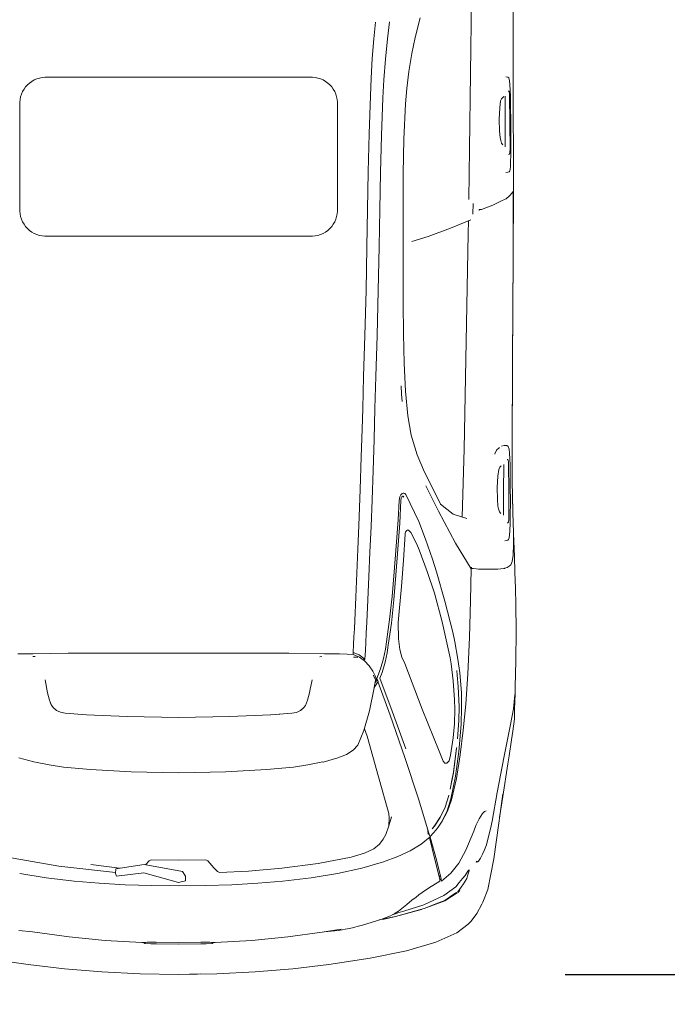
# Model space of a CAD drawing. Units: millimetres. Extents: x 595116 to 630915, y 909473 to 920225.
# Tile 6 of 134: x 629349 to 629404, y 919194 to 919279. Entities that reach past the tile are written whole.
import ezdxf

# ---------------------------------------------------------------- set-up
doc = ezdxf.new("R2010")
doc.units = ezdxf.units.MM
doc.layers.add('C-PRKG-VEHI', color=8, linetype='Continuous', lineweight=13)
doc.layers.add('Dimension', color=3, linetype='Continuous', lineweight=18)
doc.styles.get("Standard").update_dxf_attribs({"font": 'arial.ttf'})
doc.dimstyles.new('ISO-25', dxfattribs={"dimtxt": 9, "dimasz": 6, "dimexe": 1.25, "dimexo": 0.625, "dimtad": 1, "dimlunit": 4, "dimtxsty": 'Standard', "dimcen": 2.5, "dimadec": 0, "dimazin": 0, "dimtfac": 1, "dimtmove": 0, "dimatfit": 3, "dimfxl": 1, "dimarcsym": 0})

# ---------------------------------------------------------------- blocks, each defined once
blk = doc.blocks.new('A$C7ADB3080')
for p, q in [((1717.5, 1836.5), (2187.9, 1837.4)), ((2187.9, 1837.4), (2484.5, 1837.8)), ((2193.4, 1826), (2191.2, 1823.4)), ((2200.6, 1827.9), (2193.4, 1826)), ((2210.5, 1828.9), (2200.6, 1827.9)), ((2224.9, 1829.7), (2210.5, 1828.9)), ((2224.9, 1829.7), (2241, 1830)), ((2227.3, 1826.2), (2226.9, 1824.2)), ((2227.3, 1826.2), (2228.5, 1826.8)), ((2229.6, 1827.1), (2228.5, 1826.8)), ((2232.9, 1827.6), (2229.6, 1827.1)), ((2237.6, 1827.8), (2232.9, 1827.6)), ((2309.4, 1828.6), (2237.6, 1827.8)), ((2241, 1830), (2270.8, 1830.6)), ((2270.8, 1830.6), (2301.2, 1830.8)), ((2301.2, 1830.8), (2330.4, 1831.1)), ((2377.2, 1829.1), (2309.4, 1828.6)), ((2330.4, 1831.1), (2346.2, 1831.1)), ((2346.2, 1831.1), (2361.6, 1831.1)), ((2361.6, 1831.1), (2390.1, 1830.9)), ((2382.2, 1828.9), (2377.2, 1829.1)), ((2386.2, 1828.5), (2382.2, 1828.9)), ((2388.4, 1827.8), (2386.2, 1828.5)), ((2386.8, 1828.4), (2387.6, 1828.3)), ((2387.6, 1828.3), (2389.6, 1827.5)), ((2389.6, 1827.5), (2388.4, 1827.8)), ((2389.6, 1827.5), (2389.9, 1825.3)), ((2411.1, 1830.5), (2390.1, 1830.9)), ((2420.6, 1830), (2411.1, 1830.5)), ((2428.8, 1829.1), (2420.6, 1830)), ((2432.5, 1828.1), (2428.8, 1829.1)), ((2434.5, 1826.7), (2432.5, 1828.1)), ((2435.7, 1823.3), (2434.5, 1826.7)), ((2494.5, 1829.3), (2484.5, 1837.8)), ((2484.8, 1837.6), (2652.6, 1836.8)), ((2485.1, 1837.3), (2485.3, 1837.5)), ((2485.3, 1837.5), (2485.4, 1837.5)), ((2654.1, 1836.7), (2485.4, 1837.5)), ((2496.6, 1827.5), (2494.5, 1829.3)), ((2503.9, 1818.7), (2496.6, 1827.5)), ((2652.6, 1836.8), (2920.1, 1835.4)), ((2925, 1835.1), (2654.1, 1836.7)), ((3154.5, 1834.7), (2920.1, 1835.4)), ((2925, 1835.1), (3140.2, 1834.4)), ((3140.2, 1834.4), (3154.5, 1834.3)), ((3155.1, 1834.3), (3141.2, 1834.3)), ((3141.2, 1834.3), (3141.2, 1834.3)), ((3148.6, 1826.5), (3141.5, 1824)), ((3158.6, 1827.8), (3148.6, 1826.5)), ((3154.5, 1834.7), (3189.7, 1834.5)), ((3167.6, 1834.3), (3155.1, 1834.3)), ((3173, 1828.6), (3158.6, 1827.8)), ((3167.2, 1834.3), (3179.8, 1834.4)), ((3173, 1828.6), (3189, 1829)), ((3177.6, 1824.3), (3176.5, 1824)), ((3180.9, 1824.9), (3177.6, 1824.3)), ((3179.8, 1834.4), (3189.8, 1834.5)), ((3185.7, 1825.1), (3180.9, 1824.9)), ((3257.4, 1825.6), (3185.7, 1825.1)), ((3189, 1829), (3218.8, 1829.6)), ((3189.7, 1834.5), (3230.4, 1834.5)), ((3218.8, 1829.6), (3249.2, 1829.8)), ((3269.2, 1835.3), (3230.4, 1834.5)), ((3249.2, 1829.8), (3278.5, 1830)), ((3325.3, 1825.8), (3257.4, 1825.6)), ((3311.5, 1836.1), (3269.2, 1835.3)), ((3278.5, 1830), (3294.3, 1829.9)), ((3290.9, 1836.5), (3285.7, 1835.6)), ((3301, 1836.5), (3290.9, 1836.5)), ((3290.9, 1836.5), (3301, 1836.5)), ((3294.3, 1829.9), (3309.6, 1829.8)), ((3323.5, 1836.5), (3301, 1836.5)), ((3301, 1836.5), (3323.5, 1836.5)), ((3309.6, 1829.8), (3338.2, 1829.4)), ((3363.4, 1837.9), (3311.5, 1836.1)), ((3330.2, 1825.6), (3325.3, 1825.8)), ((3334.3, 1825.1), (3330.2, 1825.6)), ((3336.4, 1824.3), (3334.3, 1825.1)), ((3334.5, 1825), (3335.7, 1824.9)), ((3335.7, 1824.9), (3337.6, 1824)), ((3337.6, 1824), (3336.4, 1824.3)), ((3359.1, 1828.7), (3338.2, 1829.4)), ((3368.6, 1828), (3359.1, 1828.7)), ((3392, 1838.1), (3363.4, 1837.9)), ((3365.8, 1837.9), (3365.3, 1837.9)), ((3424.7, 1840.3), (3365.8, 1837.9)), ((3376.8, 1826.8), (3368.6, 1828)), ((3380.5, 1825.5), (3376.8, 1826.8)), ((3382.5, 1823.5), (3380.5, 1825.5)), ((3420.9, 1836.7), (3392, 1838.1)), ((3437.5, 1834.4), (3420.9, 1836.7)), ((3465.3, 1841.8), (3424.7, 1840.3)), ((3445.8, 1830.9), (3437.5, 1834.4)), ((3445.8, 1830.9), (3449.9, 1827.1)), ((3449.9, 1827.1), (3453.1, 1821.8)), ((3506.8, 1843), (3465.3, 1841.8)), ((3548.4, 1843.9), (3506.8, 1843)), ((3615.8, 1844.5), (3548.4, 1843.9)), ((3693.3, 1843.9), (3615.8, 1844.5)), ((3760.4, 1842.6), (3693.3, 1843.9)), ((3760.4, 1842.6), (3777.5, 1842)), ((3780.6, 1841.8), (3777.5, 1842)), ((3817.8, 1840.9), (3777.6, 1842)), ((3777.6, 1842), (3784.7, 1841.8)), ((3816.5, 1837.6), (3780.6, 1841.8)), ((3856.8, 1830), (3816.5, 1837.6)), ((3842, 1840.1), (3817.8, 1840.9)), ((3873.8, 1836.4), (3842, 1840.1)), ((3938.8, 1813.9), (3856.8, 1830)), ((3896.2, 1832.9), (3873.8, 1836.4)), ((3896.2, 1832.9), (3937.3, 1826.5)), ((3937.3, 1826.5), (3958, 1823.1)), ((2190.4, 1818.3), (2191.2, 1823.4)), ((2240, 1816.8), (2309.6, 1816.6)), ((2243.3, 1810.5), (2241.1, 1813.1)), ((2246.7, 1807.3), (2243.3, 1810.5)), ((2252.5, 1804.7), (2246.7, 1807.3)), ((2270.3, 1802.6), (2252.5, 1804.7)), ((2299.3, 1801.5), (2270.3, 1802.6)), ((2330.4, 1802), (2299.3, 1801.5)), ((2309.6, 1816.6), (2370.7, 1816.9)), ((2346.9, 1803.3), (2330.4, 1802)), ((2354, 1805), (2346.9, 1803.3)), ((2361.4, 1807), (2354, 1805)), ((2365.7, 1810.3), (2361.4, 1807)), ((2436.2, 1818.2), (2435.7, 1823.3)), ((2504.3, 1818.2), (2503.9, 1818.7)), ((2505, 1816.9), (2504.3, 1818.2)), ((2510.7, 1805), (2505, 1816.9)), ((2520.5, 1784.5), (2510.7, 1805)), ((3138.8, 1818), (3139.2, 1820.6)), ((3138.8, 1816.6), (3138.9, 1817.6)), ((3139.2, 1812.5), (3138.8, 1816.6)), ((3141.5, 1824), (3139.2, 1820.6)), ((3139.6, 1808.8), (3139.6, 1809.6)), ((3140.7, 1807.1), (3139.6, 1808.8)), ((3143.9, 1801.9), (3143.8, 1801.9)), ((3151.3, 1793.8), (3143.9, 1801.9)), ((3175.3, 1823.4), (3174.9, 1821.4)), ((3175.3, 1823.4), (3176.5, 1824)), ((3187.9, 1813.2), (3257.6, 1812.5)), ((3194.7, 1802.6), (3191.3, 1806.1)), ((3200.5, 1799.8), (3194.7, 1802.6)), ((3218.3, 1797.4), (3200.5, 1799.8)), ((3257.6, 1812.5), (3318.7, 1812.5)), ((3301.9, 1799.5), (3294.9, 1797.7)), ((3309.3, 1801.6), (3301.9, 1799.5)), ((3313.6, 1805.2), (3309.3, 1801.6)), ((3337.6, 1824), (3338, 1821.8)), ((3383.7, 1819.1), (3382.5, 1823.5)), ((3384, 1816), (3383.7, 1819.1)), ((3453.1, 1821.8), (3454.9, 1815.7)), ((3454.9, 1815.7), (3455.1, 1815)), ((3455.1, 1815), (3455.4, 1813.2)), ((3455.4, 1813.2), (3456.9, 1797.4)), ((4032, 1795.9), (3938.8, 1813.9)), ((3958, 1823.1), (4042.4, 1810.1)), ((4110.6, 1799.9), (4035.1, 1810.4)), ((4035.2, 1810.4), (4035.1, 1810.4)), ((4042.4, 1810.1), (4096.4, 1801.8)), ((4202.8, 1787.5), (4110.6, 1799.9)), ((2532.1, 1755.6), (2520.5, 1784.5)), ((3160.5, 1789.8), (3151.3, 1793.8)), ((3161.6, 1789.6), (3160.5, 1789.8)), ((3247.2, 1796.1), (3218.3, 1797.4)), ((3278.4, 1796.4), (3247.2, 1796.1)), ((3294.9, 1797.7), (3278.4, 1796.4)), ((3456.9, 1797.4), (3456.9, 1768.6)), ((4106, 1782.7), (4032, 1795.9)), ((4125.1, 1778.5), (4106, 1782.7)), ((4145.5, 1773.8), (4125.1, 1778.5)), ((4166.8, 1768.8), (4145.5, 1773.8)), ((4281.2, 1771.5), (4202.8, 1787.5)), ((2532.1, 1755.6), (2532.1, 1749.2)), ((2533.9, 1749.8), (2532.1, 1749.8)), ((2534.6, 1749.8), (2533.9, 1749.8)), ((3454.3, 1729.9), (3456.9, 1748.3)), ((3456.9, 1768.6), (3456.9, 1748.3)), ((4080, 1765.6), (4079.5, 1767.9)), ((4081, 1763.4), (4079.8, 1766.2)), ((4082.5, 1761.6), (4081, 1763.4)), ((4086.1, 1758.5), (4082.5, 1761.6)), ((4099.9, 1749.3), (4086.1, 1758.5)), ((4116.9, 1741.3), (4099.9, 1749.3)), ((4179.6, 1763.4), (4166.8, 1768.8)), ((4190.3, 1758.6), (4179.6, 1763.4)), ((4201, 1753), (4190.3, 1758.6)), ((4208.9, 1748.3), (4201, 1753)), ((4208.9, 1748.3), (4210.6, 1746.2)), ((4314.2, 1759.2), (4281.2, 1771.5)), ((4314.2, 1759.2), (4319.2, 1756.8)), ((4343.6, 1743.2), (4319.2, 1756.8)), ((2375.6, 1724.9), (1724.4, 1733.1)), ((2506, 1723.1), (2375.6, 1724.9)), ((2543.4, 1733.4), (2516.3, 1733.9)), ((2579.5, 1676.2), (2558, 1728.1)), ((3456.6, 1729.3), (3390, 1688.5)), ((3455.3, 1729.9), (3452.5, 1730)), ((3452.6, 1726.9), (3455.5, 1729.2)), ((3455.3, 1729.2), (3455.3, 1733.4)), ((3455.3, 1728.5), (3455.3, 1729)), ((3537.8, 1727.6), (3456.6, 1729.3)), ((3632.9, 1724.7), (3537.8, 1727.6)), ((3726.9, 1720.6), (3632.9, 1724.7)), ((4131.6, 1736.2), (4116.9, 1741.3)), ((4180, 1714.9), (4131.6, 1736.2)), ((4208.9, 1742.4), (4210.6, 1746.2)), ((4211.3, 1742.1), (4209, 1742.8)), ((4210, 1745), (4210.4, 1744.8)), ((4210.4, 1744.8), (4211.4, 1741.7)), ((4230.6, 1723.8), (4234.6, 1720.4)), ((4233.3, 1723.8), (4230.6, 1723.8)), ((4234.6, 1720.4), (4230.6, 1723.8)), ((4230.6, 1723.8), (4233.3, 1723.8)), ((4246.7, 1719.9), (4233.3, 1723.8)), ((4233.3, 1723.8), (4246.7, 1719.9)), ((4343.6, 1743.2), (4363.1, 1729.2)), ((4370.3, 1721.1), (4363.1, 1729.2)), ((2594.2, 1721.7), (2560.4, 1722.3)), ((3148.3, 1710.7), (2594.2, 1721.7)), ((3323, 1705.8), (3148.3, 1710.7)), ((3327.1, 1717.9), (3315.3, 1682.8)), ((3724.3, 1699.5), (3689.1, 1694.4)), ((3689.1, 1694.4), (3724.3, 1699.5)), ((3774.5, 1703.9), (3724.3, 1699.5)), ((3724.3, 1699.5), (3774.5, 1703.9)), ((3804.6, 1715.3), (3726.9, 1720.6)), ((3759.2, 1696), (3811.2, 1697.9)), ((3812.3, 1704.6), (3774.5, 1703.9)), ((3774.5, 1703.9), (3812.3, 1704.6)), ((3871.4, 1708.8), (3804.6, 1715.3)), ((3811.2, 1697.9), (3846.5, 1697)), ((3856.9, 1703.3), (3812.3, 1704.6)), ((3812.3, 1704.6), (3856.9, 1703.3)), ((3926.7, 1697.5), (3856.9, 1703.3)), ((3856.9, 1703.3), (3926.7, 1697.5)), ((3935.4, 1700.8), (3871.4, 1708.8)), ((3990.3, 1688.8), (3926.7, 1697.5)), ((3926.7, 1697.5), (3990.3, 1688.8)), ((3995.6, 1690.9), (3935.4, 1700.8)), ((4213.7, 1697), (4180, 1714.9)), ((4234.6, 1720.4), (4245.3, 1713.2)), ((4245.3, 1713.2), (4234.6, 1720.4)), ((4245.3, 1713.2), (4253.1, 1706.5)), ((4253.1, 1706.5), (4245.3, 1713.2)), ((4252.8, 1717.5), (4246.7, 1719.9)), ((4246.7, 1719.9), (4252.8, 1717.5)), ((4259.8, 1713.6), (4252.8, 1717.5)), ((4252.8, 1717.5), (4259.8, 1713.6)), ((4253.1, 1706.5), (4263.7, 1698)), ((4263.7, 1698), (4253.1, 1706.5)), ((4266.7, 1709.2), (4259.8, 1713.6)), ((4259.8, 1713.6), (4266.7, 1709.2)), ((4263.7, 1698), (4274.7, 1689.4)), ((4274.7, 1689.4), (4263.7, 1698)), ((4275.4, 1703.2), (4266.7, 1709.2)), ((4266.7, 1709.2), (4275.4, 1703.2)), ((4287.1, 1694.7), (4275.4, 1703.2)), ((4275.4, 1703.2), (4287.1, 1694.7)), ((4288.8, 1695.5), (4283, 1700)), ((4370.3, 1721.1), (4392.6, 1692.2)), ((2601.1, 1618), (2579.5, 1676.2)), ((3315.3, 1682.8), (3289.8, 1650.3)), ((3390, 1688.5), (3307.9, 1644.8)), ((3619.1, 1681.8), (3540, 1661.1)), ((3540, 1661.1), (3619.1, 1681.8)), ((3592.6, 1654.4), (3685.5, 1675.3)), ((3685.5, 1675.3), (3592.6, 1654.4)), ((3644.1, 1687), (3619.1, 1681.8)), ((3619.1, 1681.8), (3644.1, 1687)), ((3689.1, 1694.4), (3644.1, 1687)), ((3644.1, 1687), (3689.1, 1694.4)), ((3685.5, 1675.3), (3701, 1677.9)), ((3701, 1677.9), (3685.5, 1675.3)), ((3701, 1677.9), (3744.9, 1682.9)), ((3744.9, 1682.9), (3701, 1677.9)), ((3718.4, 1692), (3730.4, 1693.4)), ((3730.4, 1693.4), (3759.2, 1696)), ((3744.9, 1682.9), (3793.1, 1686.4)), ((3793.1, 1686.4), (3744.9, 1682.9)), ((3793.1, 1686.4), (3817.7, 1687.2)), ((3817.7, 1687.2), (3793.1, 1686.4)), ((3817.7, 1687.2), (3854.8, 1686)), ((3854.8, 1686), (3817.7, 1687.2)), ((3846.5, 1697), (3893.4, 1693.5)), ((3854.8, 1686), (3891.3, 1682.8)), ((3891.3, 1682.8), (3854.8, 1686)), ((3891.3, 1682.8), (3936.2, 1676.3)), ((3936.2, 1676.3), (3891.3, 1682.8)), ((3916.3, 1691.8), (3917.5, 1691.7)), ((3979.7, 1683.5), (3917.3, 1691.7)), ((3917.5, 1691.7), (3981.3, 1683.4)), ((3936.2, 1676.3), (3950.2, 1672.4)), ((3950.2, 1672.4), (3936.2, 1676.3)), ((3950.2, 1672.4), (3956.1, 1666.6)), ((3956.1, 1666.6), (3950.2, 1672.4)), ((4004.3, 1678.6), (3979.7, 1683.5)), ((3981.3, 1683.4), (4023.5, 1674.8)), ((4048.1, 1677.1), (3990.3, 1688.8)), ((3990.3, 1688.8), (4048.1, 1677.1)), ((4050.7, 1678.1), (3995.6, 1690.9)), ((4010.7, 1677.4), (4004.3, 1678.6)), ((4078.8, 1667.3), (4048.1, 1677.1)), ((4048.1, 1677.1), (4078.8, 1667.3)), ((4050.7, 1678.1), (4080.1, 1667.8)), ((4050.7, 1678.1), (4050.7, 1678.1)), ((4080.1, 1667.8), (4050.7, 1678.1)), ((4239.6, 1677.1), (4213.7, 1697)), ((4260.4, 1652.9), (4239.6, 1677.1)), ((4274.7, 1689.4), (4297.1, 1658.8)), ((4297.1, 1658.8), (4274.7, 1689.4)), ((4290.4, 1690), (4287.1, 1694.7)), ((4287.1, 1694.7), (4290.4, 1690)), ((4310.5, 1661.7), (4290.3, 1693.3)), ((4301.5, 1673.7), (4290.4, 1690)), ((4290.4, 1690), (4301.5, 1673.7)), ((4309.4, 1661.5), (4301.5, 1673.7)), ((4301.5, 1673.7), (4309.4, 1661.5)), ((4392.6, 1692.2), (4416.8, 1638.5)), ((3289.8, 1650.3), (3201.4, 1606)), ((3540, 1661.1), (3463.8, 1640.1)), ((3463.8, 1640.1), (3540, 1661.1)), ((3519.3, 1634.8), (3592.6, 1654.4)), ((3592.6, 1654.4), (3519.3, 1634.8)), ((3951.6, 1657.2), (3925.2, 1646.4)), ((3925.2, 1646.4), (3951.6, 1657.2)), ((3956, 1661.6), (3951.6, 1657.2)), ((3951.6, 1657.2), (3956, 1661.6)), ((3956.1, 1666.6), (3956, 1661.6)), ((3956, 1661.6), (3956.1, 1666.6)), ((4038.4, 1671.7), (4039.3, 1671.5)), ((4039.3, 1671.5), (4069.8, 1662)), ((4095.5, 1649.7), (4069.3, 1662.1)), ((4069.8, 1662), (4096.4, 1649.5)), ((4106, 1654.5), (4078.8, 1667.3)), ((4078.8, 1667.3), (4106, 1654.5)), ((4080.1, 1667.8), (4106, 1654.5)), ((4106, 1654.5), (4080.1, 1667.8)), ((4117.9, 1634.7), (4095.5, 1649.7)), ((4096.4, 1649.5), (4118.4, 1634.8)), ((4121, 1644.1), (4106, 1654.5)), ((4106, 1654.5), (4120.9, 1644.2)), ((4248.1, 1646.9), (4204.1, 1635.6)), ((4204.9, 1639.5), (4250.9, 1650.7)), ((4246.7, 1649.7), (4249, 1647.1)), ((4256.1, 1648.5), (4248.1, 1646.9)), ((4250.9, 1650.7), (4260.4, 1652.9)), ((4254.1, 1651.5), (4256.3, 1648.9)), ((4256.5, 1648.5), (4256.1, 1648.5)), ((4256.3, 1648.9), (4256.6, 1648.3)), ((4259.7, 1648.5), (4257.4, 1648.5)), ((4278, 1619.2), (4259.7, 1648.5)), ((4297.1, 1658.8), (4321.2, 1607.2)), ((4321.2, 1607.2), (4297.1, 1658.8)), ((4316, 1644.7), (4309.4, 1661.5)), ((4309.4, 1661.5), (4316, 1644.7)), ((4330.7, 1608.4), (4310.5, 1661.7)), ((3307.9, 1644.8), (3242.4, 1612.3)), ((3431.3, 1629.6), (3380.1, 1611.8)), ((3380.1, 1611.8), (3431.3, 1629.6)), ((3463.8, 1640.1), (3431.3, 1629.6)), ((3431.3, 1629.6), (3463.8, 1640.1)), ((3463.6, 1615.6), (3519.3, 1634.8)), ((3519.3, 1634.8), (3463.6, 1615.6)), ((3925.2, 1646.4), (3817.2, 1603)), ((3817.2, 1603), (3925.2, 1646.4)), ((4050.4, 1594.4), (4142.2, 1622)), ((4125.2, 1628.3), (4117.9, 1634.7)), ((4118.4, 1634.8), (4125.2, 1628.5)), ((4120.9, 1644.2), (4121.2, 1644)), ((4128, 1639.3), (4121.3, 1643.9)), ((4125.2, 1628.5), (4125, 1628.4)), ((4136.9, 1631), (4128, 1639.3)), ((4134.8, 1633), (4134.9, 1633)), ((4134.9, 1633), (4145.3, 1623.3)), ((4145.3, 1623.3), (4136.9, 1631)), ((4146.3, 1623.6), (4139.4, 1620.9)), ((4140.8, 1621.4), (4140.7, 1621.5)), ((4146.3, 1623.6), (4164.8, 1600.2)), ((4146.5, 1623.3), (4204.9, 1639.5)), ((4204.1, 1635.6), (4147.6, 1621.9)), ((4330, 1607.9), (4316, 1644.7)), ((4316, 1644.7), (4330, 1607.9)), ((4416.8, 1638.5), (4439, 1562.7)), ((2088.8, 1585.4), (2038.3, 1598.2)), ((2614.2, 1576.1), (2601.1, 1618)), ((3201.4, 1606), (3163.1, 1589.7)), ((3380.1, 1611.8), (3334.6, 1594.5)), ((3334.6, 1594.5), (3380.1, 1611.8)), ((3407.4, 1595.4), (3463.6, 1615.6)), ((3463.6, 1615.6), (3407.4, 1595.4)), ((3817.2, 1603), (3700.4, 1558.4)), ((3700.4, 1558.4), (3817.2, 1603)), ((4138.6, 1618.2), (4124.8, 1616.8)), ((4139.4, 1620.9), (4137.7, 1619.3)), ((4138.9, 1617.7), (4137.7, 1619.3)), ((4164.8, 1600.2), (4181.7, 1572.2)), ((4289.5, 1603), (4278, 1619.2)), ((4295.4, 1594.5), (4289.5, 1603)), ((4321.2, 1607.2), (4337.1, 1555.5)), ((4337.1, 1555.5), (4321.2, 1607.2)), ((4350.6, 1534.3), (4330, 1607.9)), ((4330, 1607.9), (4350.6, 1534.3)), ((4351.4, 1534.4), (4332.7, 1601.5)), ((2130.1, 1576.2), (2088.8, 1585.4)), ((2176.5, 1568.6), (2130.1, 1576.2)), ((3112.6, 1574.6), (3062.7, 1566.3)), ((3163.1, 1589.7), (3112.6, 1574.6)), ((3334.6, 1594.5), (3264.7, 1561.2)), ((3264.7, 1561.2), (3334.6, 1594.5)), ((3357.5, 1569.1), (3363.1, 1573.8)), ((3363.1, 1573.8), (3357.5, 1569.1)), ((3363.1, 1573.8), (3392.8, 1588.9)), ((3392.8, 1588.9), (3363.1, 1573.8)), ((3392.8, 1588.9), (3407.4, 1595.4)), ((3407.4, 1595.4), (3392.8, 1588.9)), ((3941.5, 1558.3), (4050.4, 1594.4)), ((4181.7, 1572.2), (4196.9, 1540)), ((4301.5, 1587.2), (4295.4, 1594.5)), ((4309, 1576.5), (4301.5, 1587.2)), ((4319.8, 1563.6), (4309, 1576.5)), ((2220.1, 1563.2), (2176.5, 1568.6)), ((2260.3, 1559.8), (2220.1, 1563.2)), ((2350.4, 1555.7), (2260.3, 1559.8)), ((2439.2, 1554), (2350.4, 1555.7)), ((2529.7, 1553.9), (2439.2, 1554)), ((2589.2, 1554.1), (2529.7, 1553.9)), ((2589.2, 1554.1), (2618.6, 1554.3)), ((2589.2, 1554.1), (2589.2, 1554.1)), ((2622.6, 1554.3), (2618.6, 1554.3)), ((2773, 1554.3), (2622.6, 1554.3)), ((2851.6, 1554.7), (2773, 1554.3)), ((2926.8, 1556.4), (2851.6, 1554.7)), ((2999.6, 1560.1), (2926.8, 1556.4)), ((3006.7, 1549.4), (2985.7, 1548.6)), ((3062.7, 1566.3), (2999.6, 1560.1)), ((3025.6, 1551.6), (3006.7, 1549.4)), ((3262.5, 1558.7), (3261.6, 1556.1)), ((3261.6, 1556.1), (3262.5, 1558.7)), ((3261.6, 1556.1), (3261.6, 1553.9)), ((3261.6, 1553.9), (3261.6, 1556.1)), ((3261.6, 1556.1), (3261.6, 1555.9)), ((3261.6, 1553.9), (3262.3, 1551.6)), ((3262.3, 1551.6), (3261.6, 1553.9)), ((3262.2, 1551.8), (3262.3, 1551.6)), ((3262.3, 1551.6), (3265.7, 1548.2)), ((3265.7, 1548.2), (3262.3, 1551.6)), ((3264.7, 1561.2), (3262.5, 1558.7)), ((3262.5, 1558.7), (3264.7, 1561.2)), ((3265.7, 1548.2), (3271, 1545.4)), ((3271, 1545.4), (3265.7, 1548.2)), ((3271, 1550.8), (3269.2, 1553.1)), ((3269.5, 1552.8), (3269.6, 1553.9)), ((3269.6, 1553.9), (3272.3, 1555.5)), ((3274.3, 1549.1), (3271, 1550.8)), ((3280.2, 1548.2), (3274.3, 1549.1)), ((3338.5, 1545.3), (3280.2, 1548.2)), ((3356.4, 1565.7), (3357.5, 1569.1)), ((3357.5, 1569.1), (3356.4, 1565.7)), ((3357.6, 1563.2), (3356.4, 1565.7)), ((3356.4, 1565.7), (3357.6, 1563.2)), ((3360.3, 1560.6), (3357.6, 1563.2)), ((3357.6, 1563.2), (3360.3, 1560.6)), ((3364.2, 1559.4), (3360.3, 1560.6)), ((3360.3, 1560.6), (3360.8, 1560.5)), ((3360.3, 1560.6), (3364.2, 1559.4)), ((3366.9, 1559), (3364.2, 1559.4)), ((3364.2, 1559.4), (3366.9, 1559)), ((3366.7, 1559.1), (3366.9, 1559)), ((3434.5, 1554.7), (3366.9, 1559)), ((3366.9, 1559), (3434.5, 1554.7)), ((3501.9, 1549.7), (3434.5, 1554.7)), ((3434.5, 1554.7), (3501.9, 1549.7)), ((3566, 1543.9), (3501.9, 1549.7)), ((3501.9, 1549.7), (3566, 1543.9)), ((3683.7, 1550.7), (3664.1, 1545.3)), ((3664.1, 1545.3), (3683.7, 1550.7)), ((3700.4, 1558.4), (3683.7, 1550.7)), ((3683.7, 1550.7), (3700.4, 1558.4)), ((3919.8, 1561.3), (3822.4, 1525.6)), ((3832.9, 1520.5), (3941.5, 1558.3)), ((4337.2, 1542.2), (4319.8, 1563.6)), ((4337.1, 1555.5), (4341.1, 1543)), ((4341.1, 1543), (4337.1, 1555.5)), ((4439, 1562.7), (4458.5, 1469.5)), ((3271, 1545.4), (3280.2, 1543.8)), ((3280.2, 1543.8), (3271, 1545.4)), ((3280.2, 1543.8), (3330.4, 1541.1)), ((3330.4, 1541.1), (3280.2, 1543.8)), ((3330.4, 1541.1), (3397.7, 1536.4)), ((3397.7, 1536.4), (3330.4, 1541.1)), ((3405.7, 1540.6), (3338.5, 1545.3)), ((3397.7, 1536.4), (3464.1, 1531.2)), ((3464.1, 1531.2), (3397.7, 1536.4)), ((3472.6, 1535.6), (3405.7, 1540.6)), ((3464.1, 1531.2), (3527.2, 1525.6)), ((3527.2, 1525.6), (3464.1, 1531.2)), ((3536, 1530), (3472.6, 1535.6)), ((3527.2, 1525.6), (3587, 1519.2)), ((3587, 1519.2), (3527.2, 1525.6)), ((3596.5, 1523.8), (3536, 1530)), ((3594.2, 1541.4), (3566, 1543.9)), ((3566, 1543.9), (3594.2, 1541.4)), ((3636.8, 1542), (3594.2, 1541.4)), ((3594.2, 1541.4), (3636.8, 1542)), ((3653.1, 1515.9), (3596.5, 1523.8)), ((3664.1, 1545.3), (3636.8, 1542)), ((3636.8, 1542), (3664.1, 1545.3)), ((3822.4, 1525.6), (3738.1, 1493.8)), ((3746.6, 1489.3), (3832.9, 1520.5)), ((4094.2, 1524.4), (4096.2, 1523.8)), ((4094.2, 1524.4), (4117.8, 1517.2)), ((4196.9, 1540), (4210.5, 1503.8)), ((4342.8, 1533.4), (4337.2, 1542.2)), ((4341.1, 1543), (4344.1, 1534.3)), ((4344.1, 1534.3), (4341.1, 1543)), ((4348.9, 1521.9), (4342.8, 1533.4)), ((4344.1, 1534.3), (4345.7, 1528.8)), ((4345.7, 1528.8), (4344.1, 1534.3)), ((4345.7, 1528.8), (4346.6, 1526.2)), ((4346.6, 1526.2), (4345.7, 1528.8)), ((4357.7, 1499.3), (4348.9, 1521.9)), ((4359.8, 1492.7), (4350.6, 1534.3)), ((4350.6, 1534.3), (4359.8, 1492.7)), ((4358.6, 1501.7), (4351.4, 1534.4)), ((2092.8, 1514), (2048.5, 1519)), ((2048.5, 1519), (2092.8, 1514)), ((2145.3, 1508.8), (2092.8, 1514)), ((2092.8, 1514), (2145.3, 1508.8)), ((2197.8, 1504.5), (2145.3, 1508.8)), ((2145.3, 1508.8), (2197.8, 1504.5)), ((2244.2, 1501.9), (2197.8, 1504.5)), ((2197.8, 1504.5), (2244.2, 1501.9)), ((2341, 1498.7), (2244.2, 1501.9)), ((2244.2, 1501.9), (2341, 1498.7)), ((2436.5, 1496), (2341, 1498.7)), ((2341, 1498.7), (2436.5, 1496)), ((2531.6, 1493.8), (2436.5, 1496)), ((2436.5, 1496), (2531.6, 1493.8)), ((3587, 1519.2), (3643.8, 1511.6)), ((3643.8, 1511.6), (3587, 1519.2)), ((3643.8, 1511.6), (3662.7, 1508.4)), ((3662.7, 1508.4), (3643.8, 1511.6)), ((3672.4, 1512.7), (3653.1, 1515.9)), ((3662.7, 1508.4), (3687.1, 1503.5)), ((3687.1, 1503.5), (3662.7, 1508.4)), ((3696.9, 1507.4), (3672.4, 1512.7)), ((3687.1, 1503.5), (3713.6, 1496.2)), ((3713.6, 1496.2), (3687.1, 1503.5)), ((3723.1, 1499.8), (3696.9, 1507.4)), ((3713.6, 1496.2), (3716.2, 1495.2)), ((3738.7, 1486.4), (3713.6, 1496.2)), ((3738.1, 1493.8), (3723.1, 1499.8)), ((3991.5, 1490.9), (4085.9, 1517)), ((4085.9, 1517), (3991.5, 1490.9)), ((4085.9, 1517), (4096.8, 1518.2)), ((4096.8, 1518.2), (4085.9, 1517)), ((4096.8, 1518.2), (4117.8, 1517.2)), ((4117.8, 1517.2), (4096.8, 1518.2)), ((4117.8, 1517.2), (4140.4, 1509.4)), ((4140.4, 1509.4), (4117.8, 1517.2)), ((4140.4, 1509.4), (4152.4, 1502.3)), ((4152.4, 1502.3), (4140.4, 1509.4)), ((4152.4, 1502.3), (4165, 1492.8)), ((4165, 1492.8), (4152.4, 1502.3)), ((4210.5, 1503.8), (4227, 1447.4)), ((4365.6, 1474.4), (4357.7, 1499.3)), ((2049.5, 1482.6), (2093, 1478.3)), ((2093, 1478.3), (2049.5, 1482.6)), ((2093, 1478.3), (2143.5, 1474.7)), ((2143.5, 1474.7), (2093, 1478.3)), ((2143.5, 1474.7), (2194, 1471.9)), ((2194, 1471.9), (2143.5, 1474.7)), ((2194, 1471.9), (2239.7, 1470.1)), ((2239.7, 1470.1), (2194, 1471.9)), ((2239.7, 1470.1), (2337.4, 1467)), ((2337.4, 1467), (2239.7, 1470.1)), ((2627.7, 1492.2), (2531.6, 1493.8)), ((2531.6, 1493.8), (2627.7, 1492.2)), ((2739.8, 1490), (2627.7, 1492.2)), ((2627.7, 1492.2), (2739.8, 1490)), ((2855.6, 1486.9), (2739.8, 1490)), ((2739.8, 1490), (2855.6, 1486.9)), ((2961.5, 1483.8), (2855.6, 1486.9)), ((2855.6, 1486.9), (2961.5, 1483.8)), ((3043.6, 1481.5), (2961.5, 1483.8)), ((2961.5, 1483.8), (3043.6, 1481.5)), ((3123.9, 1479.4), (3043.6, 1481.5)), ((3043.6, 1481.5), (3123.9, 1479.4)), ((3203.4, 1477), (3123.9, 1479.4)), ((3123.9, 1479.4), (3203.4, 1477)), ((3279, 1474.4), (3203.4, 1477)), ((3203.4, 1477), (3279, 1474.4)), ((3347.7, 1471.6), (3279, 1474.4)), ((3279, 1474.4), (3347.7, 1471.6)), ((3413.9, 1468.6), (3347.7, 1471.6)), ((3347.7, 1471.6), (3413.9, 1468.6)), ((3719.7, 1476), (3706.1, 1467)), ((3733.7, 1482.6), (3719.7, 1476)), ((3730.8, 1477.9), (3730, 1477.5)), ((3741.7, 1483.1), (3730.8, 1477.9)), ((3743.8, 1486.4), (3733.7, 1482.6)), ((3736.9, 1487.1), (3738.7, 1486.4)), ((3738.2, 1493.8), (3738.1, 1493.8)), ((3746.3, 1489.5), (3738.5, 1486.3)), ((3738.5, 1486.3), (3739.1, 1484.6)), ((3738.7, 1486.4), (3740.1, 1486.9)), ((3738.7, 1486.3), (3738.7, 1486.4)), ((3738.7, 1484.5), (3738.7, 1485.8)), ((3748.7, 1481.8), (3741.7, 1483.1)), ((3749.9, 1481.6), (3743.8, 1486.4)), ((3746.3, 1489.5), (3762, 1479.9)), ((3755.7, 1480.5), (3748.7, 1481.8)), ((3762.8, 1479.3), (3755.7, 1480.5)), ((3762, 1479.9), (3762.7, 1479.3)), ((3821.6, 1467.4), (3762.8, 1479.3)), ((3887, 1461.1), (3991.5, 1490.9)), ((3991.5, 1490.9), (3887, 1461.1)), ((4165, 1492.8), (4176.6, 1478.3)), ((4176.6, 1478.3), (4165, 1492.8)), ((4176.6, 1478.3), (4188.1, 1454.7)), ((4188.1, 1454.7), (4176.6, 1478.3)), ((4373.8, 1446.9), (4365.6, 1474.4)), ((4474.9, 1362.7), (4458.5, 1469.5)), ((2337.4, 1467), (2434.6, 1464.3)), ((2434.6, 1464.3), (2337.4, 1467)), ((2434.6, 1464.3), (2531.7, 1462.2)), ((2531.7, 1462.2), (2434.6, 1464.3)), ((2531.7, 1462.2), (2628.6, 1460.7)), ((2628.6, 1460.6), (2531.7, 1462.2)), ((2628.6, 1460.7), (2740.5, 1458.5)), ((2740.5, 1458.5), (2628.6, 1460.6)), ((2628.8, 1460.7), (2628.8, 1460.6)), ((2740.5, 1458.5), (2856, 1455.4)), ((2856, 1455.4), (2740.5, 1458.5)), ((2856, 1455.4), (2961.6, 1452.4)), ((2961.6, 1452.4), (2856, 1455.4)), ((2961.6, 1452.4), (3043.5, 1450.2)), ((3043.5, 1450.2), (2961.6, 1452.4)), ((3043.5, 1450.2), (3097.4, 1448.7)), ((3097.4, 1448.7), (3043.5, 1450.2)), ((3097.4, 1448.7), (3168.2, 1446.4)), ((3168.2, 1446.4), (3097.4, 1448.7)), ((3168.2, 1446.4), (3252, 1443.4)), ((3252, 1443.4), (3168.2, 1446.4)), ((3476.6, 1465.7), (3413.9, 1468.6)), ((3413.9, 1468.6), (3476.6, 1465.7)), ((3536.4, 1463), (3476.6, 1465.7)), ((3476.6, 1465.7), (3536.4, 1463)), ((3593.8, 1460.5), (3536.4, 1463)), ((3536.4, 1463), (3593.8, 1460.5)), ((3622.3, 1459.2), (3593.8, 1460.5)), ((3593.8, 1460.5), (3622.3, 1459.2)), ((3645.7, 1457.9), (3622.3, 1459.2)), ((3622.3, 1459.2), (3645.7, 1457.9)), ((3666.9, 1456.8), (3645.7, 1457.9)), ((3645.7, 1457.9), (3666.9, 1456.8)), ((3688.7, 1455.7), (3666.9, 1456.8)), ((3666.9, 1456.8), (3688.7, 1455.7)), ((3677.3, 1440.6), (3688.7, 1455.7)), ((3692.8, 1454.4), (3683.5, 1441.6)), ((3688.7, 1453.7), (3687.2, 1453.8)), ((3688.7, 1455.7), (3691.7, 1452.8)), ((3689.8, 1454.7), (3688.7, 1453.7)), ((3706.1, 1467), (3692.8, 1454.4)), ((3872.7, 1453.3), (3821.6, 1467.4)), ((3868.3, 1454.5), (3887, 1461.1)), ((3887, 1461.1), (3868.3, 1454.5)), ((3910.3, 1437.3), (3872.7, 1453.3)), ((4188.1, 1454.7), (4198, 1420.7)), ((4198, 1420.7), (4188.1, 1454.7)), ((4227, 1447.4), (4240.7, 1384.8)), ((4376, 1438.7), (4373.8, 1446.9)), ((3252, 1443.4), (3344.7, 1439.9)), ((3344.7, 1439.9), (3252, 1443.4)), ((3344.7, 1439.9), (3405.5, 1437.5)), ((3405.5, 1437.5), (3344.7, 1439.9)), ((3405.5, 1437.5), (3467.2, 1434.9)), ((3467.2, 1434.9), (3405.5, 1437.5)), ((3467.2, 1434.9), (3528.9, 1432.2)), ((3528.9, 1432.2), (3467.2, 1434.9)), ((3528.9, 1432.2), (3589.5, 1429.6)), ((3589.5, 1429.6), (3528.9, 1432.2)), ((3589.5, 1429.6), (3610.4, 1428.6)), ((3610.4, 1428.6), (3589.5, 1429.6)), ((3610.4, 1428.6), (3631.1, 1427.6)), ((3631.1, 1427.6), (3610.4, 1428.6)), ((3631.1, 1427.6), (3651.3, 1426.7)), ((3651.3, 1426.7), (3631.1, 1427.6)), ((3651.3, 1426.7), (3671.3, 1425.7)), ((3671.3, 1425.7), (3651.3, 1426.7)), ((3671.3, 1425.7), (3677.3, 1440.6)), ((3676.4, 1425.9), (3671.3, 1425.7)), ((3676.4, 1425.7), (3675.9, 1409.8)), ((3683.5, 1441.6), (3676.4, 1425.7)), ((3683.8, 1435.6), (3683.3, 1426.1)), ((3684.4, 1437.3), (3683.8, 1435.6)), ((3923.1, 1425.6), (3910.3, 1437.3)), ((3933.8, 1407.9), (3923.1, 1425.6)), ((4198, 1420.7), (4214.9, 1335.7)), ((4214.9, 1335.7), (4198, 1420.7)), ((4379.1, 1427.3), (4376, 1438.7)), ((4381.9, 1416.3), (4379.1, 1427.3)), ((3675.9, 1409.8), (3675.4, 1390)), ((3942.9, 1386), (3933.8, 1407.9)), ((4382.9, 1411.3), (4381.9, 1416.3)), ((4383.8, 1405.1), (4382.9, 1411.3)), ((4383.4, 1394.3), (4391.4, 1346)), ((4385.2, 1397), (4383.8, 1405.1)), ((4386.9, 1387.2), (4385.2, 1397)), ((2263, 1385.3), (2528.8, 1385.3)), ((2395.9, 1385.3), (2466.3, 1385.3)), ((3675.1, 1370.7), (3674.7, 1351.3)), ((3675.4, 1390), (3675.1, 1370.7)), ((3953.5, 1347.9), (3942.9, 1386)), ((4240.7, 1384.8), (4251.7, 1317)), ((4386.9, 1387.2), (4390.5, 1351.5)), ((3674.7, 1351.3), (3673.7, 1260.2)), ((3682.1, 1344.7), (3682.8, 1339.8)), ((3961.1, 1308.5), (3953.3, 1347.8)), ((4391.4, 1346), (4403.4, 1257.3)), ((4485.4, 1269.9), (4474.9, 1362.7)), ((3770, 1314.4), (3741.9, 1319.7)), ((4214.9, 1335.7), (4227, 1242)), ((4227, 1242), (4214.9, 1335.7)), ((2191, 1313.5), (2191, 639.5)), ((2600.7, 1313.5), (2600.7, 639.5)), ((3775.6, 1312.9), (3765.8, 1315.1)), ((3794, 1307.7), (3775.6, 1312.9)), ((3801.6, 1305.4), (3794, 1307.7)), ((3807.7, 1302.5), (3801.6, 1305.4)), ((3813.6, 1298.2), (3807.7, 1302.5)), ((3820.8, 1290.2), (3813.6, 1298.2)), ((3820.9, 1289.8), (3818.1, 1293.1)), ((3966.3, 1272), (3961.1, 1308.5)), ((4251.7, 1317), (4260.1, 1244.8)), ((3825.7, 1280.1), (3820.9, 1289.8)), ((3828.2, 1267.8), (3825.7, 1280.1)), ((3832.1, 1214), (3828.2, 1267.8)), ((3972.7, 1202.5), (3966.3, 1272)), ((4493.2, 1173.2), (4485.4, 1269.9)), ((3673.7, 1260.2), (3673.2, 1159.8)), ((4227, 1242), (4233.9, 1156.3)), ((4233.9, 1156.3), (4227, 1242)), ((4260.1, 1244.8), (4265.5, 1180.1)), ((4403.4, 1257.3), (4412.5, 1164.9)), ((3832, 1212.9), (3830.5, 1236.6)), ((3836.6, 1108.1), (3832, 1212.9)), ((3978.7, 1098.1), (3972.7, 1202.5)), ((4265.5, 1180.1), (4269.2, 1113.4)), ((4498.2, 1074.5), (4493.2, 1173.2)), ((3673.2, 1159.8), (3673.1, 1061.9)), ((4233.9, 1156.3), (4237.4, 1081.3)), ((4237.4, 1081.3), (4233.9, 1156.3)), ((4412.5, 1164.9), (4418.1, 1070.5)), ((3838.8, 976.2), (3836.6, 1108.1)), ((3981.5, 976.2), (3978.7, 1098.1)), ((4269.2, 1113.4), (4271.3, 1045.3)), ((4225.5, 1067.1), (4207.4, 1051.7)), ((4207.4, 1051.7), (4225.5, 1067.1)), ((4235.5, 1076.1), (4225.5, 1067.1)), ((4225.5, 1067.1), (4235.5, 1076.1)), ((4237.4, 1081.3), (4235.5, 1076.1)), ((4235.5, 1076.1), (4237.4, 1081.3)), ((4417.7, 1062.1), (4418.2, 1065.7)), ((4418.4, 1065.3), (4417.7, 1060.7)), ((4418.1, 1070.5), (4418.2, 1066)), ((4418.2, 1065.7), (4418.2, 1066)), ((4420.5, 1062.9), (4418.4, 1065.3)), ((4499.9, 976.2), (4498.2, 1074.5)), ((3673.1, 1061.9), (3673.4, 976.2)), ((4207.4, 1051.7), (4204.9, 1046.5)), ((4204.9, 1046.5), (4207.4, 1051.7)), ((4204.9, 1046.5), (4206.1, 976.2)), ((4206.1, 976.2), (4204.9, 1046.5)), ((4271.3, 1045.3), (4272, 976.2)), ((4417, 1042.8), (4417.1, 1050.5)), ((4417.1, 1048.9), (4417, 1042.1)), ((4417.1, 1033.3), (4417, 1042.8)), ((4417.1, 1050.5), (4417.4, 1056.8)), ((4417.4, 1054.8), (4417.1, 1048.9)), ((4417.4, 1056.8), (4417.7, 1062.1)), ((4417.7, 1060.7), (4417.4, 1054.8)), ((4420.5, 1062.9), (4421, 1047.5)), ((4421, 1047.5), (4421.4, 1033.2)), ((4418.2, 976.2), (4417.1, 1033.3)), ((4422.2, 976.2), (4421.4, 1033.2)), ((4500, 976.2), (4498.9, 1032.6)), ((4247.3, 994.5), (4234.9, 986.8)), ((4247.3, 994.5), (4259.3, 994)), ((4259.3, 994), (4263.7, 976.4)), ((3673.4, 976.2), (3673.1, 890.5)), ((3836.6, 844.3), (3838.8, 976.2)), ((3978.7, 854.2), (3981.5, 976.2)), ((4206.1, 976.2), (4204.9, 905.9)), ((4204.9, 905.9), (4206.1, 976.2)), ((4234.9, 986.8), (4217.4, 887.5)), ((4263.7, 976.4), (4238.2, 886.7)), ((4272, 976.2), (4271.3, 907.1)), ((4417.1, 919.1), (4418.2, 976.2)), ((4421.4, 919.2), (4422.2, 976.2)), ((4498.2, 877.8), (4500, 976.2)), ((4417, 909.5), (4417.1, 919.1)), ((4421.4, 919.2), (4421, 904.9)), ((3673.1, 890.5), (3673.2, 792.6)), ((4204.9, 905.9), (4207.4, 900.7)), ((4207.4, 900.7), (4204.9, 905.9)), ((4207.4, 900.7), (4218.1, 891.5)), ((4218.1, 891.5), (4207.4, 900.7)), ((4217.4, 887.5), (4228.4, 814.6)), ((4271.3, 907.1), (4269.2, 839)), ((4417, 910.2), (4417.1, 903.4)), ((4417.1, 901.9), (4417, 909.5)), ((4417.1, 903.4), (4417.4, 897.5)), ((4417.4, 895.6), (4417.1, 901.9)), ((4417.4, 897.5), (4417.7, 892.2)), ((4417.7, 890.3), (4417.4, 895.6)), ((4417.7, 892.2), (4418.4, 887.1)), ((4418.2, 886.7), (4417.7, 890.3)), ((4418.4, 887.1), (4420.5, 889.6)), ((4421, 904.9), (4420.5, 889.6)), ((4238.2, 886.7), (4246.8, 816.9)), ((4418.1, 881.9), (4412.5, 787.5)), ((4418.2, 886.4), (4418.1, 881.9)), ((4418.2, 886.4), (4418.2, 886.7)), ((4493.2, 779.2), (4498.2, 877.8)), ((3832, 739.5), (3836.6, 844.3)), ((3972.7, 749.9), (3978.7, 854.2)), ((4269.2, 839), (4265.5, 772.3)), ((4226.9, 824.6), (4217.1, 750.8)), ((4221.8, 668.4), (4237.6, 814.2)), ((4228.4, 814.6), (4240.3, 814.1)), ((4246.8, 816.9), (4240.3, 814.1)), ((3673.2, 792.6), (3673.7, 692.2)), ((4412.5, 787.5), (4403.4, 695.1)), ((4265.5, 772.3), (4260.1, 707.5)), ((4485.4, 682.5), (4493.2, 779.2)), ((3828.2, 684.6), (3832, 739.5)), ((3966.3, 680.4), (3972.7, 749.9)), ((3673.7, 692.2), (3674.7, 601.1)), ((3825.6, 672.2), (3828.2, 684.6)), ((4260.1, 707.5), (4251.7, 635.4)), ((4403.4, 695.1), (4390.5, 600.8)), ((3813.4, 654), (3820.8, 662.4)), ((3820.7, 662), (3825.6, 672.2)), ((3961, 643.5), (3966.3, 680.4)), ((4195.1, 515.6), (4221.8, 668.4)), ((4474.9, 589.7), (4485.4, 682.5)), ((3741.9, 632.7), (3775.6, 639.5)), ((3775.6, 639.5), (3794, 644.6)), ((3794, 644.6), (3801.5, 647)), ((3800.8, 646.4), (3807.5, 649.8)), ((3801.5, 647), (3806, 649)), ((3807.5, 649.8), (3813.4, 654)), ((3953.3, 603.8), (3961, 643.5)), ((4251.7, 635.4), (4240.7, 567.6)), ((3674.7, 601.1), (3675.1, 581.7)), ((3682.1, 607.7), (3682.1, 601.7)), ((3942.5, 565.4), (3953.3, 603.8)), ((4390.5, 600.8), (4386.9, 565.1)), ((4458.5, 482.9), (4474.9, 589.7)), ((2263, 567.7), (2528.8, 567.7)), ((3675.1, 581.7), (3675.4, 562.4))]:
    blk.add_line(p, q)
for centre, start, end in [((2259.6, 1316.8), 87.1848, 182.6876), ((2532.2, 1316.8), 357.3124, 92.8152), ((2259.6, 636.3), 177.3124, 272.8152), ((2532.2, 636.3), 267.1848, 2.6876)]:
    blk.add_arc(centre, 68.6, start, end)
blk = doc.blocks.new('*D186')
at = {"layer": 'Defpoints', "color": 0, "transparency": 16777216}
for p in [(629394.93, 919347.236), (629394.93, 919196.66), (629417.516, 919196.66)]:
    blk.add_point(p, dxfattribs=at)
at = {"layer": 'Dimension', "color": 0, "lineweight": -2, "transparency": 16777216}
for p, q in [((629395.555, 919347.236), (629418.766, 919347.236)), ((629417.516, 919341.236), (629417.516, 919202.66)), ((629395.555, 919196.66), (629418.766, 919196.66))]:
    blk.add_line(p, q, dxfattribs=at)
at = {"layer": 'Dimension', "color": 0, "transparency": 16777216}
for points in [[(629416.516, 919341.236), (629418.516, 919341.236), (629417.516, 919347.236)], [(629416.516, 919202.66), (629418.516, 919202.66), (629417.516, 919196.66)]]:
    blk.add_solid(points, dxfattribs=at)
at = {"layer": 'Dimension', "color": 0, "transparency": 16777216, "insert": (629412.238, 919271.948), "char_height": 9, "attachment_point": 5, "rotation": 90}
blk.add_mtext('CAR 12\'-6 1/2" TYP.', dxfattribs=at)
blk = doc.blocks.new('*D215')
at = {"layer": 'Defpoints', "color": 0, "transparency": 16777216}
for p in [(629316.041, 919411.828), (629505.041, 919411.828), (629505.041, 918832.378)]:
    blk.add_point(p, dxfattribs=at)
at = {"layer": 'Dimension', "color": 0, "lineweight": -2, "transparency": 16777216}
for p, q in [((629316.041, 919411.203), (629316.041, 918831.128)), ((629505.041, 919411.203), (629505.041, 918831.128)), ((629322.041, 918832.378), (629499.041, 918832.378))]:
    blk.add_line(p, q, dxfattribs=at)
at = {"layer": 'Dimension', "color": 0, "transparency": 16777216}
for points in [[(629322.041, 918833.378), (629322.041, 918831.378), (629316.041, 918832.378)], [(629499.041, 918833.378), (629499.041, 918831.378), (629505.041, 918832.378)]]:
    blk.add_solid(points, dxfattribs=at)
at = {"layer": 'Dimension', "color": 0, "transparency": 16777216, "insert": (629410.541, 918837.598), "char_height": 9, "attachment_point": 5}
blk.add_mtext('15\'-9"', dxfattribs=at)
blk = doc.blocks.new('*D221')
at = {"layer": 'Defpoints', "color": 0, "transparency": 16777216}
for p in [(629511.274, 919302.009), (629155.382, 919160.917), (629511.274, 919160.917)]:
    blk.add_point(p, dxfattribs=at)
at = {"layer": 'Dimension', "color": 0, "lineweight": -2, "transparency": 16777216}
for p, q in [((629510.649, 919302.009), (629154.132, 919302.009)), ((629155.382, 919296.009), (629155.382, 919166.917)), ((629510.649, 919160.917), (629154.132, 919160.917))]:
    blk.add_line(p, q, dxfattribs=at)
at = {"layer": 'Dimension', "color": 0, "transparency": 16777216}
for points in [[(629154.382, 919296.009), (629156.382, 919296.009), (629155.382, 919302.009)], [(629154.382, 919166.917), (629156.382, 919166.917), (629155.382, 919160.917)]]:
    blk.add_solid(points, dxfattribs=at)
at = {"layer": 'Dimension', "color": 0, "transparency": 16777216, "insert": (629150.162, 919231.463), "char_height": 9, "attachment_point": 5, "rotation": 90}
blk.add_mtext('11\'-9"', dxfattribs=at)

msp = doc.modelspace()

# ---------------------------------------------------------------- block references
at = {"layer": 'C-PRKG-VEHI', "xscale": 0.0334614614063694, "yscale": 0.0334614614063694, "zscale": 0.0334614614063694, "rotation": 270}
msp.add_blockref('A$C7ADB3080', (629329.6, 919347.236), dxfattribs=at)

# ---------------------------------------------------------------- dimensions: what is measured, and where the dimension line sits
at = {"layer": 'Dimension'}
dim = msp.add_linear_dim(base=(629505.041, 918832.378), p1=(629316.041, 919411.828), p2=(629505.041, 919411.828), dimstyle='ISO-25', override={"dimdec": 1, "dimlfac": 1, "dimrnd": 0, "dimzin": 1, "dimdsep": 46, "dimlunit": 4, "dimfrac": 2}, dxfattribs=at)
dim.commit()
dim.dimension.update_dxf_attribs({"geometry": '*D215', "text_midpoint": (629410.541, 918837.598)})
dim = msp.add_linear_dim(base=(629417.516, 919196.66), p1=(629394.93, 919347.236), p2=(629394.93, 919196.66), angle=270, text='CAR <> TYP.', dimstyle='ISO-25', override={"dimdec": 1, "dimlfac": 1, "dimrnd": 0, "dimzin": 1, "dimdsep": 46, "dimlunit": 4, "dimfrac": 2}, dxfattribs=at)
dim.commit()
dim.dimension.update_dxf_attribs({"geometry": '*D186', "text_midpoint": (629412.238, 919271.948)})
dim = msp.add_linear_dim(base=(629155.382, 919160.917), p1=(629511.274, 919302.009), p2=(629511.274, 919160.917), angle=90, dimstyle='ISO-25', override={"dimdec": 1, "dimlfac": 1, "dimrnd": 0, "dimzin": 1, "dimdsep": 46, "dimlunit": 4, "dimfrac": 2}, dxfattribs=at)
dim.commit()
dim.dimension.update_dxf_attribs({"geometry": '*D221', "text_midpoint": (629150.162, 919231.463)})

doc.saveas('drawing.dxf')
